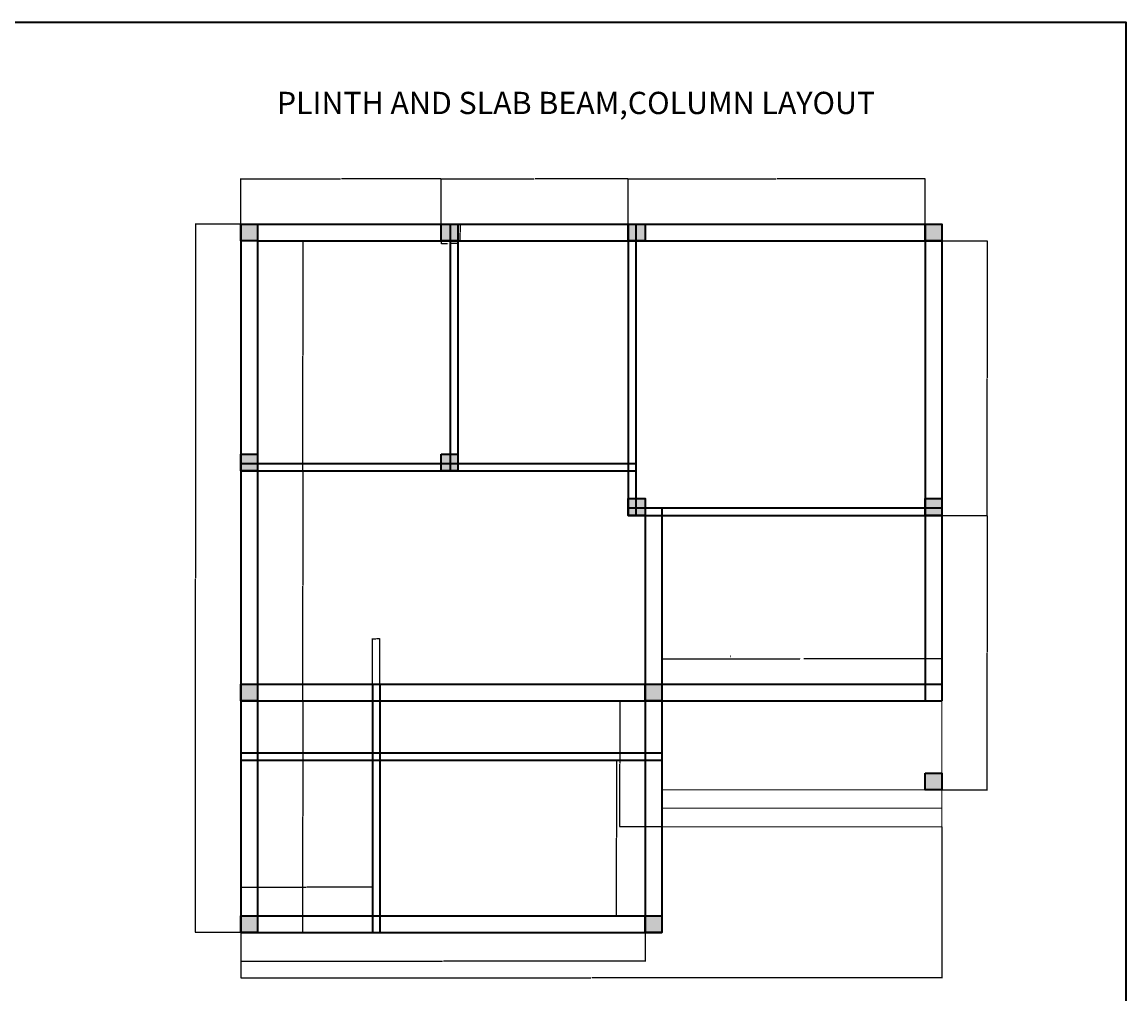
# Model space of a CAD drawing. Units: inches. Extents: x 2473 to 3664, y 1231 to 2079.
# Tile 8 of 8: x 3069 to 3664, y 1555 to 2079. Entities that reach past the tile are written whole.
import ezdxf

# ---------------------------------------------------------------- set-up
doc = ezdxf.new("R2010")
doc.units = ezdxf.units.IN
doc.linetypes.add('ACAD_ISO02W100', pattern=[15, 12, -3])
doc.layers.get('Defpoints').update_dxf_attribs({"linetype": 'ACAD_ISO02W100'})
for name, color, linetype, lineweight in [('A-ANNO-DIMS', 2, 'Continuous', 18), ('A-ANNO-TEXT', 4, 'Continuous', 25), ('A-ANNO-TTLB', 7, 'Continuous', 35), ('A-FLOR-STRS', 7, 'Continuous', 18), ('S-BEAM', 7, 'Continuous', 35), ('S-COLS', 1, 'Continuous', 35)]:
    doc.layers.add(name, color=color, linetype=linetype, lineweight=lineweight)
doc.styles.get("Standard").update_dxf_attribs({"font": 'arial.ttf'})
doc.dimstyles.get("Standard").update_dxf_attribs({"dimtxt": 0.18, "dimasz": 0.18, "dimexe": 0.18, "dimexo": 0.0625, "dimgap": 0.09, "dimtad": 0, "dimtih": 1, "dimtoh": 1, "dimdec": 4, "dimzin": 0, "dimdsep": 46, "dimtxsty": 'Standard', "dimcen": 0.09, "dimadec": 0, "dimazin": 0, "dimtfac": 1, "dimtdec": 4, "dimtofl": 0, "dimtmove": 0, "dimatfit": 3, "dimfxl": 1, "dimtolj": 1, "dimtzin": 0, "dimarcsym": 0})

# ---------------------------------------------------------------- blocks, each defined once
blk = doc.blocks.new('COL-9X9')
h = blk.add_hatch(color=256)
h.dxf.hatch_style = 1
h.paths.add_polyline_path([(9, 9), (0, 9), (0, 0), (9, 0)])
blk.add_lwpolyline([(0, 9), (9, 9), (9, 0), (0, 0)], close=True)
blk = doc.blocks.new('STEPS-SITOUT-PLAN')
for p, q in [((151, 68), (151, 0)), ((0, 20), (151, 20)), ((0, 10), (151, 10)), ((0, 0), (151, 0))]:
    blk.add_line(p, q)
blk = doc.blocks.new('*D17')
at = {"layer": 'A-ANNO-DIMS', "color": 0, "lineweight": -2, "transparency": 16777216}
for p, q in [((3294.46, 1960.99), (3294.46, 1959.53)), ((3294.64, 1959.71), (3297.93, 1959.71)), ((3303.28, 1959.71), (3300, 1959.71)), ((3303.46, 1960.99), (3303.46, 1959.53))]:
    blk.add_line(p, q, dxfattribs=at)
at = {"layer": 'A-ANNO-DIMS', "color": 0, "transparency": 16777216}
for points in [[(3294.64, 1959.74), (3294.64, 1959.68), (3294.46, 1959.71)], [(3303.28, 1959.74), (3303.28, 1959.68), (3303.46, 1959.71)]]:
    blk.add_solid(points, dxfattribs=at)
at = {"layer": 'Defpoints', "color": 0, "transparency": 16777216}
for p in [(3294.46, 1961.06), (3303.46, 1961.06), (3303.46, 1959.71)]:
    blk.add_point(p, dxfattribs=at)
at = {"layer": 'A-ANNO-DIMS', "color": 0, "transparency": 16777216, "insert": (3298.96, 1959.71), "char_height": 0.18, "attachment_point": 5}
blk.add_mtext('\\A1;COLUMN 9 TYP.', dxfattribs=at)
blk = doc.blocks.new('*D18')
at = {"layer": 'A-ANNO-DIMS', "color": 0, "lineweight": -2, "transparency": 16777216}
for p, q in [((3303.52, 1970.06), (3304.99, 1970.06)), ((3304.81, 1969.88), (3304.81, 1965.74)), ((3304.81, 1961.24), (3304.81, 1965.37)), ((3303.52, 1961.06), (3304.99, 1961.06))]:
    blk.add_line(p, q, dxfattribs=at)
at = {"layer": 'A-ANNO-DIMS', "color": 0, "transparency": 16777216}
for points in [[(3304.78, 1969.88), (3304.84, 1969.88), (3304.81, 1970.06)], [(3304.78, 1961.24), (3304.84, 1961.24), (3304.81, 1961.06)]]:
    blk.add_solid(points, dxfattribs=at)
at = {"layer": 'Defpoints', "color": 0, "transparency": 16777216}
for p in [(3303.46, 1970.06), (3304.81, 1970.06), (3303.46, 1961.06)]:
    blk.add_point(p, dxfattribs=at)
at = {"layer": 'A-ANNO-DIMS', "color": 0, "transparency": 16777216, "insert": (3304.81, 1965.56), "char_height": 0.18, "attachment_point": 5}
blk.add_mtext('\\A1;9 TYP.', dxfattribs=at)
blk = doc.blocks.new('*D35')
at = {"layer": 'A-ANNO-DIMS', "color": 0, "lineweight": -2, "transparency": 16777216}
for p, q in [((3413.46, 1713.12), (3413.46, 1735.89)), ((3413.64, 1735.71), (3487.87, 1735.71)), ((3564.28, 1735.71), (3490.06, 1735.71)), ((3564.46, 1713.12), (3564.46, 1735.89))]:
    blk.add_line(p, q, dxfattribs=at)
at = {"layer": 'A-ANNO-DIMS', "color": 0, "transparency": 16777216}
for points in [[(3413.64, 1735.74), (3413.64, 1735.68), (3413.46, 1735.71)], [(3564.28, 1735.74), (3564.28, 1735.68), (3564.46, 1735.71)]]:
    blk.add_solid(points, dxfattribs=at)
at = {"layer": 'Defpoints', "color": 0, "transparency": 16777216}
for p in [(3564.46, 1735.71), (3413.46, 1713.06), (3564.46, 1713.06)]:
    blk.add_point(p, dxfattribs=at)
at = {"layer": 'A-ANNO-DIMS', "color": 0, "transparency": 16777216, "insert": (3488.96, 1735.71), "char_height": 0.18, "attachment_point": 5}
blk.add_mtext('\\A1;SITOUT 151 TYP.', dxfattribs=at)
blk = doc.blocks.new('*D36')
at = {"layer": 'A-ANNO-DIMS', "color": 0, "lineweight": -2, "transparency": 16777216}
for p, q in [((3413.4, 1713.06), (3390.63, 1713.06)), ((3390.81, 1712.88), (3390.81, 1679.24)), ((3390.81, 1645.24), (3390.81, 1678.87)), ((3413.4, 1645.06), (3390.63, 1645.06))]:
    blk.add_line(p, q, dxfattribs=at)
at = {"layer": 'A-ANNO-DIMS', "color": 0, "transparency": 16777216}
for points in [[(3390.78, 1712.88), (3390.84, 1712.88), (3390.81, 1713.06)], [(3390.78, 1645.24), (3390.84, 1645.24), (3390.81, 1645.06)]]:
    blk.add_solid(points, dxfattribs=at)
at = {"layer": 'Defpoints', "color": 0, "transparency": 16777216}
for p in [(3390.81, 1713.06), (3413.46, 1713.06), (3413.46, 1645.06)]:
    blk.add_point(p, dxfattribs=at)
at = {"layer": 'A-ANNO-DIMS', "color": 0, "transparency": 16777216, "insert": (3390.81, 1679.06), "char_height": 0.18, "attachment_point": 5}
blk.add_mtext('\\A1;68 TYP.', dxfattribs=at)
blk = doc.blocks.new('*D65')
at = {"layer": 'A-ANNO-DIMS', "color": 0, "lineweight": -2, "transparency": 16777216}
for p, q in [((3564.46, 1644.99), (3564.46, 1563.43)), ((3186.46, 1587.99), (3186.46, 1563.43)), ((3186.64, 1563.61), (3375.17, 1563.61)), ((3564.28, 1563.61), (3375.75, 1563.61))]:
    blk.add_line(p, q, dxfattribs=at)
at = {"layer": 'A-ANNO-DIMS', "color": 0, "transparency": 16777216}
for points in [[(3186.64, 1563.64), (3186.64, 1563.58), (3186.46, 1563.61)], [(3564.28, 1563.64), (3564.28, 1563.58), (3564.46, 1563.61)]]:
    blk.add_solid(points, dxfattribs=at)
at = {"layer": 'Defpoints', "color": 0, "transparency": 16777216}
for p in [(3564.46, 1645.06), (3186.46, 1588.06), (3564.46, 1563.61)]:
    blk.add_point(p, dxfattribs=at)
at = {"layer": 'A-ANNO-DIMS', "color": 0, "transparency": 16777216, "insert": (3375.46, 1563.61), "char_height": 0.18, "attachment_point": 5}
blk.add_mtext('\\A1;378', dxfattribs=at)
blk = doc.blocks.new('*D66')
at = {"layer": 'A-ANNO-DIMS', "color": 0, "lineweight": -2, "transparency": 16777216}
for p, q in [((3186.4, 1970.06), (3161.83, 1970.06)), ((3162.01, 1969.88), (3162.01, 1779.24)), ((3162.01, 1588.24), (3162.01, 1778.87)), ((3186.4, 1588.06), (3161.83, 1588.06))]:
    blk.add_line(p, q, dxfattribs=at)
at = {"layer": 'A-ANNO-DIMS', "color": 0, "transparency": 16777216}
for points in [[(3161.98, 1969.88), (3162.04, 1969.88), (3162.01, 1970.06)], [(3161.98, 1588.24), (3162.04, 1588.24), (3162.01, 1588.06)]]:
    blk.add_solid(points, dxfattribs=at)
at = {"layer": 'Defpoints', "color": 0, "transparency": 16777216}
for p in [(3162.01, 1970.06), (3186.46, 1970.06), (3186.46, 1588.06)]:
    blk.add_point(p, dxfattribs=at)
at = {"layer": 'A-ANNO-DIMS', "color": 0, "transparency": 16777216, "insert": (3162.01, 1779.06), "char_height": 0.18, "attachment_point": 5}
blk.add_mtext('\\A1;382', dxfattribs=at)
blk = doc.blocks.new('*D67')
at = {"layer": 'A-ANNO-DIMS', "color": 0, "lineweight": -2, "transparency": 16777216}
for p, q in [((3186.46, 1970.12), (3186.46, 1994.69)), ((3186.64, 1994.51), (3240.18, 1994.51)), ((3294.28, 1994.51), (3240.74, 1994.51)), ((3294.46, 1970.12), (3294.46, 1994.69))]:
    blk.add_line(p, q, dxfattribs=at)
at = {"layer": 'A-ANNO-DIMS', "color": 0, "transparency": 16777216}
for points in [[(3186.64, 1994.54), (3186.64, 1994.48), (3186.46, 1994.51)], [(3294.28, 1994.54), (3294.28, 1994.48), (3294.46, 1994.51)]]:
    blk.add_solid(points, dxfattribs=at)
at = {"layer": 'Defpoints', "color": 0, "transparency": 16777216}
for p in [(3294.46, 1994.51), (3186.46, 1970.06), (3294.46, 1970.06)]:
    blk.add_point(p, dxfattribs=at)
at = {"layer": 'A-ANNO-DIMS', "color": 0, "transparency": 16777216, "insert": (3240.46, 1994.51), "char_height": 0.18, "attachment_point": 5}
blk.add_mtext('\\A1;108', dxfattribs=at)
blk = doc.blocks.new('*D68')
at = {"layer": 'A-ANNO-DIMS', "color": 0, "lineweight": -2, "transparency": 16777216}
for p, q in [((3294.46, 1970.12), (3294.46, 1994.69)), ((3294.64, 1994.51), (3344.7, 1994.51)), ((3395.28, 1994.51), (3345.23, 1994.51)), ((3395.46, 1970.12), (3395.46, 1994.69))]:
    blk.add_line(p, q, dxfattribs=at)
at = {"layer": 'A-ANNO-DIMS', "color": 0, "transparency": 16777216}
for points in [[(3294.64, 1994.54), (3294.64, 1994.48), (3294.46, 1994.51)], [(3395.28, 1994.54), (3395.28, 1994.48), (3395.46, 1994.51)]]:
    blk.add_solid(points, dxfattribs=at)
at = {"layer": 'Defpoints', "color": 0, "transparency": 16777216}
for p in [(3395.46, 1994.51), (3294.46, 1970.06), (3395.46, 1970.06)]:
    blk.add_point(p, dxfattribs=at)
at = {"layer": 'A-ANNO-DIMS', "color": 0, "transparency": 16777216, "insert": (3344.96, 1994.51), "char_height": 0.18, "attachment_point": 5}
blk.add_mtext('\\A1;101', dxfattribs=at)
blk = doc.blocks.new('*D69')
at = {"layer": 'A-ANNO-DIMS', "color": 0, "lineweight": -2, "transparency": 16777216}
for p, q in [((3395.46, 1970.12), (3395.46, 1994.69)), ((3395.64, 1994.51), (3475.18, 1994.51)), ((3555.28, 1994.51), (3475.74, 1994.51)), ((3555.46, 1970.12), (3555.46, 1994.69))]:
    blk.add_line(p, q, dxfattribs=at)
at = {"layer": 'A-ANNO-DIMS', "color": 0, "transparency": 16777216}
for points in [[(3395.64, 1994.54), (3395.64, 1994.48), (3395.46, 1994.51)], [(3555.28, 1994.54), (3555.28, 1994.48), (3555.46, 1994.51)]]:
    blk.add_solid(points, dxfattribs=at)
at = {"layer": 'Defpoints', "color": 0, "transparency": 16777216}
for p in [(3555.46, 1994.51), (3395.46, 1970.06), (3555.46, 1970.06)]:
    blk.add_point(p, dxfattribs=at)
at = {"layer": 'A-ANNO-DIMS', "color": 0, "transparency": 16777216, "insert": (3475.46, 1994.51), "char_height": 0.18, "attachment_point": 5}
blk.add_mtext('\\A1;160', dxfattribs=at)
blk = doc.blocks.new('*D70')
at = {"layer": 'A-ANNO-DIMS', "color": 0, "lineweight": -2, "transparency": 16777216}
for p, q in [((3195.52, 1713.06), (3220.09, 1713.06)), ((3219.91, 1712.88), (3219.91, 1650.74)), ((3219.91, 1588.24), (3219.91, 1650.37)), ((3195.52, 1588.06), (3220.09, 1588.06))]:
    blk.add_line(p, q, dxfattribs=at)
at = {"layer": 'A-ANNO-DIMS', "color": 0, "transparency": 16777216}
for points in [[(3219.88, 1712.88), (3219.94, 1712.88), (3219.91, 1713.06)], [(3219.88, 1588.24), (3219.94, 1588.24), (3219.91, 1588.06)]]:
    blk.add_solid(points, dxfattribs=at)
at = {"layer": 'Defpoints', "color": 0, "transparency": 16777216}
for p in [(3195.46, 1713.06), (3195.46, 1588.06), (3219.91, 1588.06)]:
    blk.add_point(p, dxfattribs=at)
at = {"layer": 'A-ANNO-DIMS', "color": 0, "transparency": 16777216, "insert": (3219.91, 1650.56), "char_height": 0.18, "attachment_point": 5}
blk.add_mtext('\\A1;125', dxfattribs=at)
blk = doc.blocks.new('*D71')
at = {"layer": 'A-ANNO-DIMS', "color": 0, "lineweight": -2, "transparency": 16777216}
for p, q in [((3195.52, 1837.06), (3220.09, 1837.06)), ((3219.91, 1836.88), (3219.91, 1775.24)), ((3219.91, 1713.24), (3219.91, 1774.88)), ((3195.52, 1713.06), (3220.09, 1713.06))]:
    blk.add_line(p, q, dxfattribs=at)
at = {"layer": 'A-ANNO-DIMS', "color": 0, "transparency": 16777216}
for points in [[(3219.88, 1836.88), (3219.94, 1836.88), (3219.91, 1837.06)], [(3219.88, 1713.24), (3219.94, 1713.24), (3219.91, 1713.06)]]:
    blk.add_solid(points, dxfattribs=at)
at = {"layer": 'Defpoints', "color": 0, "transparency": 16777216}
for p in [(3195.46, 1837.06), (3195.46, 1713.06), (3219.91, 1713.06)]:
    blk.add_point(p, dxfattribs=at)
at = {"layer": 'A-ANNO-DIMS', "color": 0, "transparency": 16777216, "insert": (3219.91, 1775.06), "char_height": 0.18, "attachment_point": 5}
blk.add_mtext('\\A1;124', dxfattribs=at)
blk = doc.blocks.new('*D72')
at = {"layer": 'A-ANNO-DIMS', "color": 0, "lineweight": -2, "transparency": 16777216}
for p, q in [((3195.52, 1961.06), (3220.09, 1961.06)), ((3219.91, 1960.88), (3219.91, 1899.24)), ((3219.91, 1837.24), (3219.91, 1898.88)), ((3195.52, 1837.06), (3220.09, 1837.06))]:
    blk.add_line(p, q, dxfattribs=at)
at = {"layer": 'A-ANNO-DIMS', "color": 0, "transparency": 16777216}
for points in [[(3219.88, 1960.88), (3219.94, 1960.88), (3219.91, 1961.06)], [(3219.88, 1837.24), (3219.94, 1837.24), (3219.91, 1837.06)]]:
    blk.add_solid(points, dxfattribs=at)
at = {"layer": 'Defpoints', "color": 0, "transparency": 16777216}
for p in [(3195.46, 1961.06), (3195.46, 1837.06), (3219.91, 1837.06)]:
    blk.add_point(p, dxfattribs=at)
at = {"layer": 'A-ANNO-DIMS', "color": 0, "transparency": 16777216, "insert": (3219.91, 1899.06), "char_height": 0.18, "attachment_point": 5}
blk.add_mtext('\\A1;124', dxfattribs=at)
blk = doc.blocks.new('*D73')
at = {"layer": 'A-ANNO-DIMS', "color": 0, "lineweight": -2, "transparency": 16777216}
for p, q in [((3564.52, 1961.06), (3589.09, 1961.06)), ((3588.91, 1960.88), (3588.91, 1887.24)), ((3588.91, 1813.24), (3588.91, 1886.87)), ((3564.52, 1813.06), (3589.09, 1813.06))]:
    blk.add_line(p, q, dxfattribs=at)
at = {"layer": 'A-ANNO-DIMS', "color": 0, "transparency": 16777216}
for points in [[(3588.88, 1960.88), (3588.94, 1960.88), (3588.91, 1961.06)], [(3588.88, 1813.24), (3588.94, 1813.24), (3588.91, 1813.06)]]:
    blk.add_solid(points, dxfattribs=at)
at = {"layer": 'Defpoints', "color": 0, "transparency": 16777216}
for p in [(3564.46, 1961.06), (3588.91, 1961.06), (3564.46, 1813.06)]:
    blk.add_point(p, dxfattribs=at)
at = {"layer": 'A-ANNO-DIMS', "color": 0, "transparency": 16777216, "insert": (3588.91, 1887.06), "char_height": 0.18, "attachment_point": 5}
blk.add_mtext('\\A1;148', dxfattribs=at)
blk = doc.blocks.new('*D74')
at = {"layer": 'A-ANNO-DIMS', "color": 0, "lineweight": -2, "transparency": 16777216}
for p, q in [((3564.52, 1813.06), (3589.09, 1813.06)), ((3588.91, 1812.88), (3588.91, 1739.24)), ((3588.91, 1665.24), (3588.91, 1738.87)), ((3564.52, 1665.06), (3589.09, 1665.06))]:
    blk.add_line(p, q, dxfattribs=at)
at = {"layer": 'A-ANNO-DIMS', "color": 0, "transparency": 16777216}
for points in [[(3588.88, 1812.88), (3588.94, 1812.88), (3588.91, 1813.06)], [(3588.88, 1665.24), (3588.94, 1665.24), (3588.91, 1665.06)]]:
    blk.add_solid(points, dxfattribs=at)
at = {"layer": 'Defpoints', "color": 0, "transparency": 16777216}
for p in [(3564.46, 1813.06), (3588.91, 1813.06), (3564.46, 1665.06)]:
    blk.add_point(p, dxfattribs=at)
at = {"layer": 'A-ANNO-DIMS', "color": 0, "transparency": 16777216, "insert": (3588.91, 1739.06), "char_height": 0.18, "attachment_point": 5}
blk.add_mtext('\\A1;148', dxfattribs=at)
blk = doc.blocks.new('*D75')
at = {"layer": 'A-ANNO-DIMS', "color": 0, "lineweight": -2, "transparency": 16777216}
for p, q in [((3186.46, 1596.99), (3186.46, 1572.43)), ((3404.46, 1596.99), (3404.46, 1572.43)), ((3186.64, 1572.61), (3295.17, 1572.61)), ((3404.28, 1572.61), (3295.75, 1572.61))]:
    blk.add_line(p, q, dxfattribs=at)
at = {"layer": 'A-ANNO-DIMS', "color": 0, "transparency": 16777216}
for points in [[(3186.64, 1572.64), (3186.64, 1572.58), (3186.46, 1572.61)], [(3404.28, 1572.64), (3404.28, 1572.58), (3404.46, 1572.61)]]:
    blk.add_solid(points, dxfattribs=at)
at = {"layer": 'Defpoints', "color": 0, "transparency": 16777216}
for p in [(3186.46, 1597.06), (3404.46, 1597.06), (3186.46, 1572.61)]:
    blk.add_point(p, dxfattribs=at)
at = {"layer": 'A-ANNO-DIMS', "color": 0, "transparency": 16777216, "insert": (3295.46, 1572.61), "char_height": 0.18, "attachment_point": 5}
blk.add_mtext('\\A1;218', dxfattribs=at)
blk = doc.blocks.new('*D76')
at = {"layer": 'A-ANNO-DIMS', "color": 0, "lineweight": -2, "transparency": 16777216}
for p, q in [((3186.46, 1588.12), (3186.46, 1612.69)), ((3186.64, 1612.51), (3221.76, 1612.51)), ((3257.28, 1612.51), (3222.16, 1612.51)), ((3257.46, 1588.12), (3257.46, 1612.69))]:
    blk.add_line(p, q, dxfattribs=at)
at = {"layer": 'A-ANNO-DIMS', "color": 0, "transparency": 16777216}
for points in [[(3186.64, 1612.54), (3186.64, 1612.48), (3186.46, 1612.51)], [(3257.28, 1612.54), (3257.28, 1612.48), (3257.46, 1612.51)]]:
    blk.add_solid(points, dxfattribs=at)
at = {"layer": 'Defpoints', "color": 0, "transparency": 16777216}
for p in [(3257.46, 1612.51), (3186.46, 1588.06), (3257.46, 1588.06)]:
    blk.add_point(p, dxfattribs=at)
at = {"layer": 'A-ANNO-DIMS', "color": 0, "transparency": 16777216, "insert": (3221.96, 1612.51), "char_height": 0.18, "attachment_point": 5}
blk.add_mtext('\\A1;71', dxfattribs=at)
blk = doc.blocks.new('*D77')
at = {"layer": 'A-ANNO-DIMS', "color": 0, "lineweight": -2, "transparency": 16777216}
for p, q in [((3257.46, 1722.12), (3257.46, 1746.69)), ((3257.64, 1746.51), (3259.31, 1746.51)), ((3261.28, 1746.51), (3259.61, 1746.51)), ((3261.46, 1722.12), (3261.46, 1746.69))]:
    blk.add_line(p, q, dxfattribs=at)
at = {"layer": 'A-ANNO-DIMS', "color": 0, "transparency": 16777216}
for points in [[(3257.64, 1746.54), (3257.64, 1746.48), (3257.46, 1746.51)], [(3261.28, 1746.54), (3261.28, 1746.48), (3261.46, 1746.51)]]:
    blk.add_solid(points, dxfattribs=at)
at = {"layer": 'Defpoints', "color": 0, "transparency": 16777216}
for p in [(3261.46, 1746.51), (3257.46, 1722.06), (3261.46, 1722.06)]:
    blk.add_point(p, dxfattribs=at)
at = {"layer": 'A-ANNO-DIMS', "color": 0, "transparency": 16777216, "insert": (3259.46, 1746.51), "char_height": 0.18, "attachment_point": 5}
blk.add_mtext('\\A1;4', dxfattribs=at)
blk = doc.blocks.new('*D78')
at = {"layer": 'A-ANNO-DIMS', "color": 0, "lineweight": -2, "transparency": 16777216}
for p, q in [((3413.4, 1681.06), (3388.83, 1681.06)), ((3389.01, 1680.88), (3389.01, 1639.24)), ((3389.01, 1597.24), (3389.01, 1638.87)), ((3413.4, 1597.06), (3388.83, 1597.06))]:
    blk.add_line(p, q, dxfattribs=at)
at = {"layer": 'A-ANNO-DIMS', "color": 0, "transparency": 16777216}
for points in [[(3388.98, 1680.88), (3389.04, 1680.88), (3389.01, 1681.06)], [(3388.98, 1597.24), (3389.04, 1597.24), (3389.01, 1597.06)]]:
    blk.add_solid(points, dxfattribs=at)
at = {"layer": 'Defpoints', "color": 0, "transparency": 16777216}
for p in [(3389.01, 1681.06), (3413.46, 1681.06), (3413.46, 1597.06)]:
    blk.add_point(p, dxfattribs=at)
at = {"layer": 'A-ANNO-DIMS', "color": 0, "transparency": 16777216, "insert": (3389.01, 1639.06), "char_height": 0.18, "attachment_point": 5}
blk.add_mtext('\\A1;84', dxfattribs=at)

msp = doc.modelspace()

# ---------------------------------------------------------------- linework, layer by layer
at = {"layer": 'A-ANNO-TTLB'}
msp.add_lwpolyline([(2473.2801, 2079.0861), (3663.7983, 2079.0861), (3663.7983, 1231.3065), (2473.2801, 1231.3065)], close=True, dxfattribs=at)
at = {"layer": 'S-BEAM'}
for p, q in [((3186.4622, 1970.0561), (3303.4622, 1970.0561)), ((3186.4622, 1970.0561), (3186.4622, 1588.0561)), ((3297.4622, 1970.0561), (3564.4622, 1970.0561)), ((3299.4622, 1970.0561), (3299.4622, 1837.0561)), ((3303.4622, 1970.0561), (3303.4622, 1837.0561)), ((3395.4622, 1970.0561), (3395.4622, 1813.0561)), ((3399.4622, 1970.0561), (3399.4622, 1817.0561)), ((3555.4622, 1970.0561), (3555.4622, 1713.0561)), ((3564.4622, 1970.0561), (3564.4622, 1713.0561)), ((3195.4622, 1961.0561), (3299.4622, 1961.0561)), ((3195.4622, 1961.0561), (3195.4622, 1597.0561)), ((3297.4622, 1961.0561), (3564.4622, 1961.0561)), ((3395.4622, 1961.0561), (3395.4622, 1855.0561)), ((3399.4622, 1956.0561), (3399.4622, 1855.0561)), ((3399.4622, 1956.0561), (3399.4622, 1855.0561)), ((3186.4622, 1841.0561), (3399.4622, 1841.0561)), ((3186.4622, 1837.0561), (3399.4622, 1837.0561)), ((3395.4622, 1819.0561), (3395.4622, 1813.0561)), ((3395.4622, 1819.0561), (3395.4622, 1813.0561)), ((3395.4622, 1817.0561), (3564.4622, 1817.0561)), ((3399.4622, 1819.0561), (3399.4622, 1813.0561)), ((3399.4622, 1819.0561), (3399.4622, 1813.0561)), ((3399.4622, 1819.0561), (3399.4622, 1813.0561)), ((3404.4622, 1817.0561), (3404.4622, 1685.0561)), ((3413.4622, 1817.0561), (3413.4622, 1588.0561)), ((3395.4622, 1813.0561), (3564.4622, 1813.0561)), ((3413.4622, 1780.5146), (3413.4622, 1588.0561)), ((3413.4622, 1761.0561), (3413.4622, 1665.0561)), ((3450.4622, 1737.0561), (3450.5193, 1737.0561)), ((3186.4622, 1722.0561), (3564.4622, 1722.0561)), ((3257.4622, 1722.0561), (3257.4622, 1588.0561)), ((3257.4622, 1721.0561), (3257.4622, 1717.0561)), ((3257.4622, 1721.0561), (3257.4622, 1685.0561)), ((3261.4622, 1722.0561), (3261.4622, 1588.0561)), ((3404.4622, 1722.0561), (3413.4622, 1722.0561)), ((3404.4622, 1721.0561), (3404.4622, 1597.0561)), ((3186.4622, 1713.0561), (3564.4622, 1713.0561)), ((3404.4622, 1713.0561), (3404.4622, 1588.0561)), ((3464.4622, 1713.0561), (3564.4622, 1713.0561)), ((3186.4622, 1685.0561), (3413.4622, 1685.0561)), ((3186.4622, 1681.0561), (3413.4622, 1681.0561)), ((3255.4622, 1681.0561), (3257.4622, 1681.0561)), ((3195.4622, 1597.0561), (3413.4622, 1597.0561)), ((3195.4622, 1597.0561), (3195.4622, 1588.0561)), ((3186.4622, 1588.0561), (3413.4622, 1588.0561))]:
    msp.add_line(p, q, dxfattribs=at)

# ---------------------------------------------------------------- block references
at = {"layer": 'A-FLOR-STRS'}
msp.add_blockref('STEPS-SITOUT-PLAN', (3413.4618, 1645.056), dxfattribs=at)
at = {"layer": 'S-COLS'}
for p in [(3186.462, 1961.056), (3294.462, 1961.056), (3395.462, 1961.056), (3555.462, 1961.056), (3186.462, 1837.056), (3294.462, 1837.056), (3395.462, 1813.056), (3555.462, 1813.056), (3186.462, 1713.056), (3404.462, 1713.056), (3555.462, 1665.056), (3186.462, 1588.056), (3404.462, 1588.056)]:
    msp.add_blockref('COL-9X9', p, dxfattribs=at)

# ---------------------------------------------------------------- texts
at = {"layer": 'A-ANNO-TEXT'}
msp.add_text('PLINTH AND SLAB BEAM,COLUMN LAYOUT', height=12, dxfattribs=at).set_placement((3205.9379, 2029.4693))

# ---------------------------------------------------------------- dimensions: what is measured, and where the dimension line sits
at = {"layer": 'A-ANNO-DIMS'}
for base, p1, p2, picture, middle in [((3294.4622, 1994.5061), (3186.4622, 1970.0561), (3294.4622, 1970.0561), '*D67', (3240.4622, 1994.5061)), ((3395.4622, 1994.5061), (3294.4622, 1970.0561), (3395.4622, 1970.0561), '*D68', (3344.9622, 1994.5061)), ((3555.4622, 1994.5061), (3395.4622, 1970.0561), (3555.4622, 1970.0561), '*D69', (3475.4622, 1994.5061)), ((3261.4622, 1746.5061), (3257.4622, 1722.0561), (3261.4622, 1722.0561), '*D77', (3259.4622, 1746.5061)), ((3564.4622, 1563.6061), (3186.4622, 1588.0561), (3564.4622, 1645.0561), '*D65', (3375.4622, 1563.6061)), ((3257.4622, 1612.5061), (3186.4622, 1588.0561), (3257.4622, 1588.0561), '*D76', (3221.9622, 1612.5061))]:
    dim = msp.add_linear_dim(base=base, p1=p1, p2=p2, dimstyle='Standard', override={"dimdec": 0, "dimlfac": 1, "dimrnd": 0, "dimzin": 0, "dimdsep": 46, "dimlunit": 2}, dxfattribs=at)
    dim.commit()
    dim.dimension.update_dxf_attribs({"geometry": picture, "text_midpoint": middle})
for base, p1, p2, angle, picture, middle in [((3162.0122, 1970.0561), (3186.4622, 1588.0561), (3186.4622, 1970.0561), 90, '*D66', (3162.0122, 1779.0561)), ((3219.9122, 1837.0561), (3195.4622, 1961.0561), (3195.4622, 1837.0561), 270, '*D72', (3219.9122, 1899.0561)), ((3588.9122, 1961.0561), (3564.4622, 1813.0561), (3564.4622, 1961.0561), 90, '*D73', (3588.9122, 1887.0561)), ((3219.9122, 1713.0561), (3195.4622, 1837.0561), (3195.4622, 1713.0561), 270, '*D71', (3219.9122, 1775.0561)), ((3588.9122, 1813.0561), (3564.4622, 1665.0561), (3564.4622, 1813.0561), 90, '*D74', (3588.9122, 1739.0561)), ((3219.9122, 1588.0561), (3195.4622, 1713.0561), (3195.4622, 1588.0561), 270, '*D70', (3219.9122, 1650.5561)), ((3389.0122, 1681.0561), (3413.4622, 1597.0561), (3413.4622, 1681.0561), 90, '*D78', (3389.0122, 1639.0561)), ((3186.4622, 1572.6061), (3404.4622, 1597.0561), (3186.4622, 1597.0561), 180, '*D75', (3295.4622, 1572.6061))]:
    dim = msp.add_linear_dim(base=base, p1=p1, p2=p2, angle=angle, dimstyle='Standard', override={"dimdec": 0, "dimlfac": 1, "dimrnd": 0, "dimzin": 0, "dimdsep": 46, "dimlunit": 2}, dxfattribs=at)
    dim.commit()
    dim.dimension.update_dxf_attribs({"geometry": picture, "text_midpoint": middle})
for base, p1, p2, picture, middle in [((3304.8122, 1970.0561), (3303.4622, 1961.0561), (3303.4622, 1970.0561), '*D18', (3304.8122, 1965.5561)), ((3390.8122, 1713.0561), (3413.4622, 1645.0561), (3413.4622, 1713.0561), '*D36', (3390.8122, 1679.0561))]:
    dim = msp.add_linear_dim(base=base, p1=p1, p2=p2, angle=90, text='<> TYP.', dimstyle='Standard', override={"dimdec": 0, "dimlfac": 1, "dimrnd": 0, "dimzin": 0, "dimdsep": 46, "dimlunit": 2}, dxfattribs=at)
    dim.commit()
    dim.dimension.update_dxf_attribs({"geometry": picture, "text_midpoint": middle})
for base, p1, p2, text, picture, middle in [((3303.4622, 1959.7061), (3294.4622, 1961.0561), (3303.4622, 1961.0561), 'COLUMN <> TYP.', '*D17', (3298.9622, 1959.7061)), ((3564.4622, 1735.7061), (3413.4622, 1713.0561), (3564.4622, 1713.0561), 'SITOUT <> TYP.', '*D35', (3488.9622, 1735.7061))]:
    dim = msp.add_linear_dim(base=base, p1=p1, p2=p2, text=text, dimstyle='Standard', override={"dimdec": 0, "dimlfac": 1, "dimrnd": 0, "dimzin": 0, "dimdsep": 46, "dimlunit": 2}, dxfattribs=at)
    dim.commit()
    dim.dimension.update_dxf_attribs({"geometry": picture, "text_midpoint": middle})

doc.saveas('drawing.dxf')
